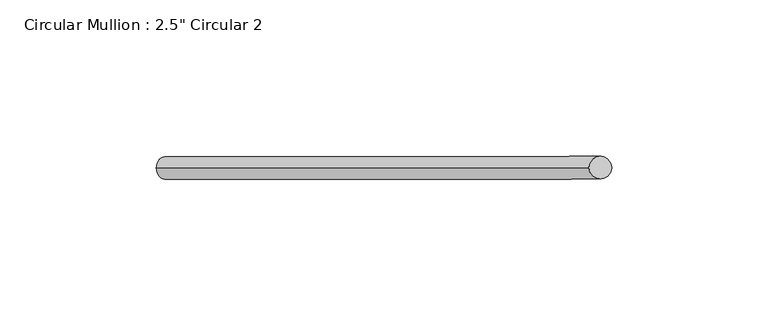
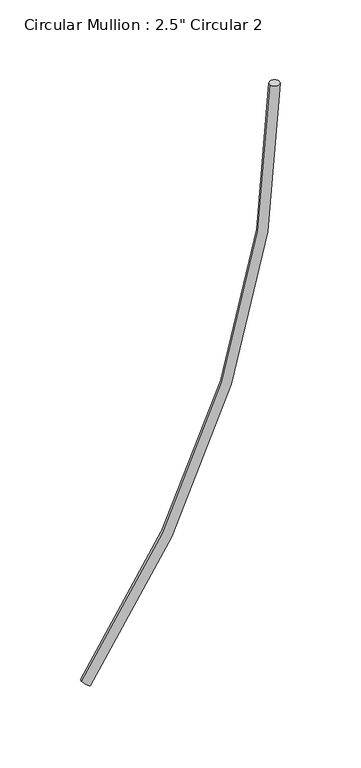
"""IFC4 building model written with IfcOpenShell, lengths in millimetres: member geometry."""

from ifc_helpers import new_model, si_unit, point, frame, origin, place, context, project, spatial, circle_curve, ellipse_curve, trimmed, source, transform, mapped, element, save
from ifc_brep_helpers import plane_surface, revolved_surface, advanced_brep


def member_ea2f4e14(model_context):
    return source(origin(), model_context, "Body", "AdvancedBrep", [
        advanced_brep(
        [(-145.4912, 0.0, -414.7566), (-7.239, 0.0, 0.0), (0.0, 0.0, 0.0), (-139.7, 0.0, -419.1)],
        [
            (0, 1, circle_curve(frame((-698.5, 0.0, 0.0), z_axis=(0.0, -1.0, 0.0), x_axis=(1.0, 0.0, 0.0)), 691.261)),
            (1, 2, circle_curve(frame((-3.6195, 0.0, 0.0), z_axis=(0.0, 0.0, -1.0), x_axis=(1.0, 0.0, 0.0)), 3.6195)),
            (2, 3, circle_curve(frame((-698.5, 0.0, 0.0), z_axis=(0.0, 1.0, 0.0), x_axis=(1.0, 0.0, 0.0)), 698.5)),
            (3, 0, circle_curve(frame((-142.5956, 0.0, -416.9283), z_axis=(0.5999999999999962, 0.0, 0.8000000000000028), x_axis=(0.8000000000000028, 0.0, -0.5999999999999962)), 3.6195)),
            (2, 1, circle_curve(frame((-3.6195, 0.0, 0.0), z_axis=(0.0, 0.0, -1.0), x_axis=(1.0, 0.0, 0.0)), 3.6195)),
            (0, 3, circle_curve(frame((-142.5956, 0.0, -416.9283), z_axis=(0.5999999999999963, 0.0, 0.8000000000000027), x_axis=(0.8000000000000027, 0.0, -0.5999999999999963)), 3.6195)),
        ],
        [
            revolved_surface(trimmed(ellipse_curve(frame((-3.6195, 0.0, 0.0), z_axis=(0.0, 0.0, 1.0), x_axis=(1.0, 0.0, 0.0)), 3.6195, 3.6195), [point((0.0, 0.0, 0.0))], [point((-7.239, 0.0, 0.0))], True, "CARTESIAN"), (-698.5, 0.0, 0.0), (0.0, 1.0, 0.0)),
            revolved_surface(trimmed(ellipse_curve(frame((-3.6195, 0.0, 0.0), z_axis=(0.0, 0.0, 1.0), x_axis=(1.0, 0.0, 0.0)), 3.6195, 3.6195), [point((-7.239, 0.0, 0.0))], [point((0.0, 0.0, 0.0))], True, "CARTESIAN"), (-698.5, 0.0, 0.0), (0.0, 1.0, 0.0)),
            plane_surface(frame((-304.8, 0.0, 0.0), z_axis=(0.0, 0.0, 1.0), x_axis=(0.0, 1.0, 0.0))),
            plane_surface(frame((104.14, 0.0, -601.98), z_axis=(-0.5999999999999963, 0.0, -0.8000000000000027), x_axis=(0.0, -1.0, 0.0))),
        ],
        [
            (0, [[1, 2, 3, 4]]),
            (1, [[-3, 5, -1, 6]]),
            (2, [[-2, -5]]),
            (3, [[-6, -4]]),
        ],
    ),
    ])


if __name__ == "__main__":
    model = new_model("IFC4")
    model_context = context("Model", 3, world=origin())
    ifc_project = project(units=[si_unit("LENGTHUNIT", "METRE", prefix="MILLI")], contexts=[model_context])
    site = spatial("IfcSite", under=ifc_project)
    building = spatial("IfcBuilding", under=site)
    placement = place(None, origin())
    member_shape = member_ea2f4e14(model_context)
    element("IfcMember", 1, ObjectType="Circular Mullion : 2.5\" Circular 2", at=placement, inside=building, context=model_context, shape_type="MappedRepresentation", body=[
        mapped(member_shape, transform((0.0, 0.0, 0.0), x_axis=(1.0, 0.0, 0.0), y_axis=(0.0, 1.0, 0.0), z_axis=(0.0, 0.0, 1.0))),
    ])
    save(model, "model.ifc")

# Revit data of these elements
# Type "Circular Mullion : 2.5\" Circular 2"
#   built-in parameter 1007350 = 0.011875 (stored number, unit not read)
# Element 1 (IfcMember, "Circular Mullion : 2.5\" Circular 2")
#   Materials on its faces: "Aluminum"
# Materials
#   "Aluminum": class "Metal", colour RGB 247 247 247, transparency 0, Description = "Aluminum 6061", Cost = 0
